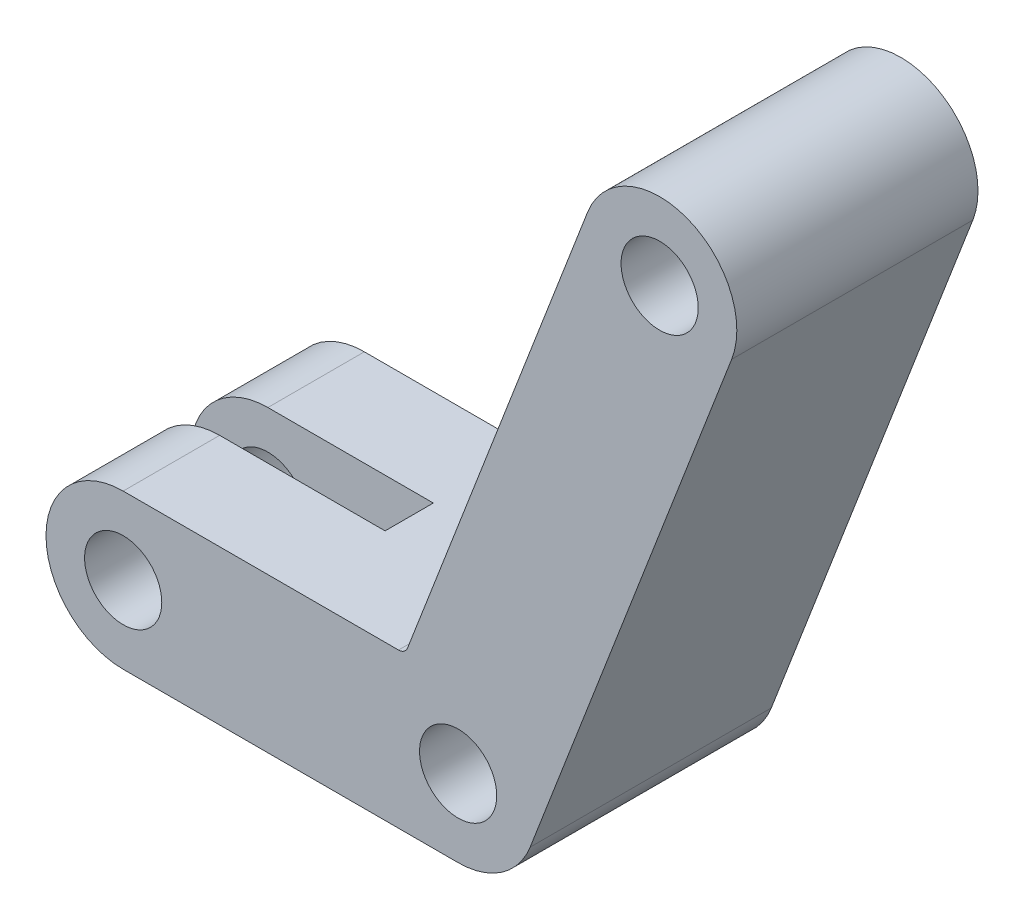
from build123d import *

# Parameters (mm, degrees)
JAW_PROFILE_SKETCH_R = 4
JAW_BODY_25MM_DEPTH  = 12.5
SLOT_SKETCH_W        = 25.15
SLOT_SKETCH_H        = 5
SLOT_CUT_5MM_DEPTH   = 25
EDGE_FILLETS_R1_R    = 1


with BuildPart() as part:
    # Jaw Profile Sketch → Jaw Body 25mm (new, symmetric)
    with BuildSketch(Plane.XY):
        with BuildLine():
            Line((24.825451548, -2.87524489), (45.715451548, 51.36475511))
            ThreePointArc((45.715451548, 51.36475511), (41.12524489, 61.705451548), (30.784548452, 57.11524489))
            Line((30.784548452, 57.11524489), (11.868297239, 8))
            Line((11.868297239, 8), (-17.36, 8))
            ThreePointArc((-17.36, 8), (-25.36, 0), (-17.36, -8))
            Line((-17.36, -8), (17.36, -8))
            ThreePointArc((17.36, -8), (21.887584393, -6.595527239), (24.825451548, -2.87524489))
        make_face()
        with Locations((38.25, 54.24)):
            Circle(JAW_PROFILE_SKETCH_R, mode=Mode.SUBTRACT)
        with Locations((-17.36, 0)):
            Circle(JAW_PROFILE_SKETCH_R, mode=Mode.SUBTRACT)
        with Locations((17.36, 0)):
            Circle(JAW_PROFILE_SKETCH_R, mode=Mode.SUBTRACT)
    extrude(amount=JAW_BODY_25MM_DEPTH, both=True)

    # Slot Sketch → Slot Cut 5mm (cut)
    with BuildSketch(Plane(origin=(0, 8, 0), x_dir=(1, 0, 0), z_dir=(0, 1, 0))):
        with Locations((-12.785, 0)):
            Rectangle(SLOT_SKETCH_W, SLOT_SKETCH_H)
    extrude(amount=-SLOT_CUT_5MM_DEPTH, mode=Mode.SUBTRACT)

    # Edge Fillets R1
    edge_fillets_r1_edges = [part.edges().sort_by_distance(p)[0] for p in [
        (11.868297239, 8, 0),
    ]]
    fillet(edge_fillets_r1_edges, radius=EDGE_FILLETS_R1_R)


solid = part.part
